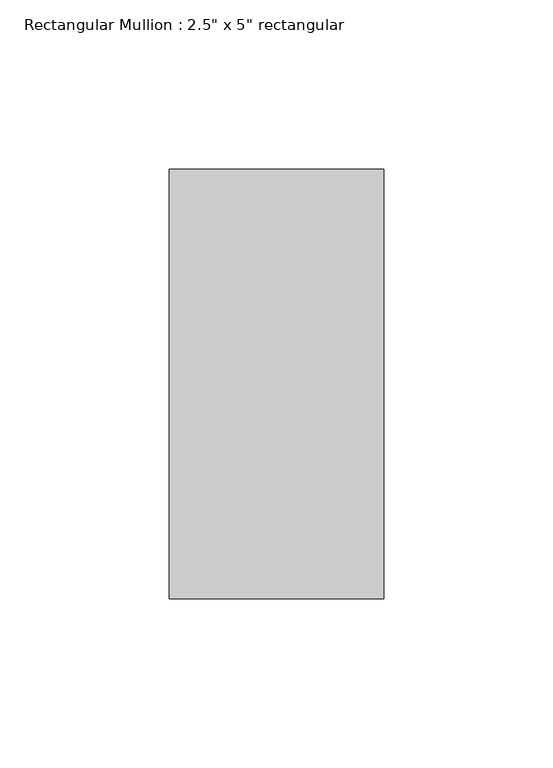
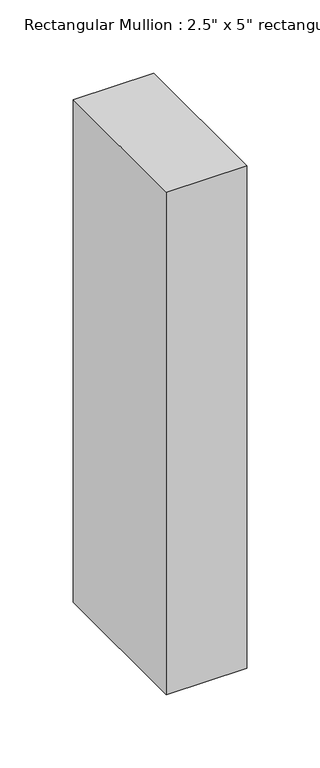
"""IFC4 building model written with IfcOpenShell, lengths in millimetres: member geometry."""

from ifc_helpers import new_model, si_unit, frame, origin, place, context, project, spatial, polyline, outline, extrude, source, transform, mapped, element, save


def member_ccaabd6e(model_context):
    return source(origin(), model_context, "Body", "SweptSolid", [
        extrude(outline(polyline([(0.0, 63.5), (0.0, -63.5), (-63.5, -63.5), (-63.5, 63.5), (0.0, 63.5)])), frame((0.0, 0.0, -419.1), z_axis=(0.0, 0.0, 1.0), x_axis=(1.0, 0.0, 0.0)), (0.0, 0.0, 1.0), 419.1),
    ])


if __name__ == "__main__":
    model = new_model("IFC4")
    model_context = context("Model", 3, world=origin())
    ifc_project = project(units=[si_unit("LENGTHUNIT", "METRE", prefix="MILLI")], contexts=[model_context])
    site = spatial("IfcSite", under=ifc_project)
    building = spatial("IfcBuilding", under=site)
    placement = place(None, origin())
    member_shape = member_ccaabd6e(model_context)
    element("IfcMember", 1, ObjectType="Rectangular Mullion : 2.5\" x 5\" rectangular", at=placement, inside=building, context=model_context, shape_type="MappedRepresentation", body=[
        mapped(member_shape, transform((0.0, 0.0, 0.0), x_axis=(1.0, 0.0, 0.0), y_axis=(0.0, 1.0, 0.0), z_axis=(0.0, 0.0, 1.0))),
    ])
    save(model, "model.ifc")

# Revit data of these elements
# Type "Rectangular Mullion : 2.5\" x 5\" rectangular"
#   built-in parameter 1007304 = 0.416667 (stored number, unit not read)
#   built-in parameter 1007301 = 0.104167 (stored number, unit not read)
#   built-in parameter 1007300 = 0.104167 (stored number, unit not read)
